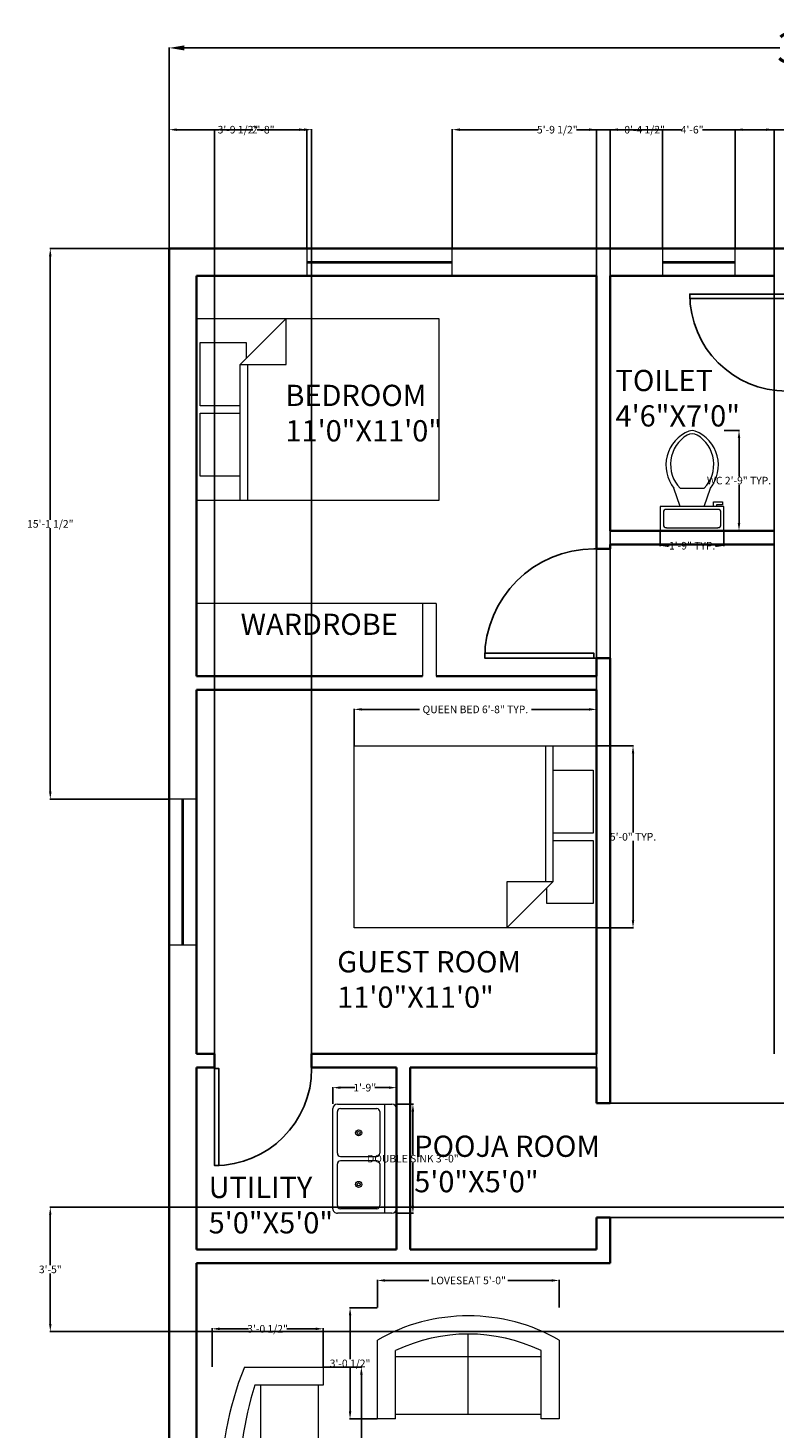
# Model space of a CAD drawing. Units: inches. Extents: x 481 to 2783, y 1975 to 3327.
# Tile 7 of 13: x 1328 to 1574, y 2866 to 3327. Entities that reach past the tile are written whole.
import ezdxf

# ---------------------------------------------------------------- set-up
doc = ezdxf.new("R2010")
doc.units = ezdxf.units.IN
doc.header["$MEASUREMENT"] = 0
for name, color, linetype, lineweight in [('A-ANNO-DIMS', 50, 'Continuous', 18), ('A-AREA-IDEN', 50, 'Continuous', 18), ('A-FLOR-CASE', 61, 'Continuous', 18), ('A-FLOR-FIXT', 61, 'Continuous', 18), ('A-FURN', 61, 'Continuous', 18), ('A-WALL', 40, 'Continuous', 35), ('DOORS', 10, 'Continuous', 25), ('WINDOWS', 220, 'Continuous', 20)]:
    doc.layers.add(name, color=color, linetype=linetype, lineweight=lineweight)
doc.styles.get("Standard").update_dxf_attribs({"font": 'arial.ttf'})
doc.dimstyles.get("Standard").update_dxf_attribs({"dimtxt": 2.5, "dimasz": 2.5, "dimexe": 0.18, "dimexo": 0.0625, "dimgap": 0.09, "dimtad": 0, "dimtih": 1, "dimtoh": 1, "dimzin": 0, "dimdsep": 46, "dimlunit": 3, "dimtxsty": 'Standard', "dimcen": 0.09, "dimadec": 0, "dimazin": 0, "dimtfac": 1, "dimtofl": 0, "dimtmove": 0, "dimatfit": 3, "dimfxl": 1, "dimtolj": 1, "dimtzin": 0, "dimarcsym": 0})

# ---------------------------------------------------------------- blocks, each defined once
blk = doc.blocks.new('*U2')
for p, q in [((0, 0), (0, -6)), ((40, 0), (40, -6))]:
    blk.add_line(p, q)
blk.add_lwpolyline([(0, 0), (0, 40), (1.75, 40), (1.75, 0)], close=True)
blk.add_arc((0, 0), 40, 0, 90)
blk = doc.blocks.new('Sink-double - 36 in top')
for p, q in [((-18, -4), (18, -4)), ((-0.75, -18.5), (-0.75, -6.5)), ((0.75, -6.5), (0.75, -18.5))]:
    blk.add_line(p, q)
for points in [[(-16.5, 0), (16.5, 0)], [(-18, -19.5), (-18, -1.5)], [(18, -1.5), (18, -19.5)], [(-16.5, -18.5), (-16.5, -6.5)], [(-15.5, -5.5), (-1.75, -5.5)], [(1.75, -5.5), (15.5, -5.5)], [(16.5, -6.5), (16.5, -18.5)], [(16.5, -21), (-16.5, -21)], [(-1.75, -19.5), (-15.5, -19.5)], [(15.5, -19.5), (1.75, -19.5)]]:
    blk.add_lwpolyline(points)
for centre, radius in [((-8.5, -12.5), 1), ((-8.5, -12.5), 0.5), ((8.5, -12.5), 1), ((8.5, -12.5), 0.5)]:
    blk.add_circle(centre, radius)
for centre, radius, start, end in [((-16.5, -1.5), 1.5, 90, 180), ((16.5, -1.5), 1.5, 0, 90), ((-15.5, -6.5), 1, 90, 180), ((-1.75, -6.5), 1, 0, 90), ((1.75, -6.5), 1, 90, 180), ((15.5, -6.5), 1, 0, 90), ((-16.5, -19.5), 1.5, 180, 270), ((-15.5, -18.5), 1, 180, 270), ((-1.75, -18.5), 1, 270, 0), ((1.75, -18.5), 1, 180, 270), ((15.5, -18.5), 1, 270, 0), ((16.5, -19.5), 1.5, 270, 0)]:
    blk.add_arc(centre, radius, start, end)
blk = doc.blocks.new('Sofa - Roundback 7 ft.')
for p, q in [((-12.00002, -32.4421), (-12.00003, -6.5971)), ((11.99997, -32.4421), (11.99998, -6.5971)), ((-36.000027, -34), (-36.000027, -11.4696)), ((-35.999844, -13.3819), (35.9998, -13.3819)), ((35.99998, -34), (35.99998, -11.4696)), ((-36.000027, -32.4421), (35.99998, -32.4421))]:
    blk.add_line(p, q)
for points in [[(-36.000027, -34), (-42.000027, -34), (-42.000027, -8)], [(41.99998, -8), (41.99998, -34), (35.99998, -34)]]:
    blk.add_lwpolyline(points)
for centre, radius, start, end in [((0, -114.25), 114.25, 68.43141, 111.5686), ((-0.00001, -127.1968), 121.1968, 72.72033, 107.2797)]:
    blk.add_arc(centre, radius, start, end)
blk = doc.blocks.new('Sofa - Roundback Loveseat 5 ft.')
for p, q in [((0, -32.44198), (0, -5.99998)), ((-24, -33.99998), (-24, -11.46958)), ((-23.9998, -13.38178), (23.99986, -13.38178)), ((24.00004, -33.99998), (24.00004, -11.46958)), ((-24, -32.44198), (24.00004, -32.44198))]:
    blk.add_line(p, q)
for points in [[(-24, -33.99998), (-30, -33.99998), (-30, -7.99998)], [(30.00004, -7.99998), (30.00004, -33.99998), (24.00004, -33.99998)]]:
    blk.add_lwpolyline(points)
for centre, radius, start, end in [((0, -60.24998), 60.24998, 60.13715, 119.8628), ((0, -61.38438), 55.38444, 64.32083, 115.6792)]:
    blk.add_arc(centre, radius, start, end)
blk = doc.blocks.new('Bed - Queen')
for p, q in [((0, -80.00003), (0, 0)), ((0, 0), (59.99999, 0)), ((59.99999, 0), (59.99999, -80.00003)), ((7.99999, -1.2), (28.79998, -1.2)), ((7.99999, -14.4), (7.99999, -1.2)), ((28.79998, -1.2), (28.79998, -14.4)), ((31.19999, -1.2), (51.99999, -1.2)), ((31.19999, -14.4), (31.19999, -1.2)), ((51.99999, -1.2), (51.99999, -16.4)), ((0, -14.4), (44.8, -14.4)), ((44.8, -16.8), (0, -16.8)), ((59.99999, -29.6), (44.8, -14.4)), ((44.8, -14.4), (44.8, -29.6)), ((51.99999, -16.4), (46.79936, -16.4)), ((44.8, -29.6), (59.99999, -29.6)), ((59.99999, -80.00003), (0, -80.00003))]:
    blk.add_line(p, q)
blk = doc.blocks.new('Toilet - top')
for p, q in [((9.5, -6), (9.5, -2)), ((-10, -8.5), (-8, -8.5)), ((-10, -9.5), (-10, -8.5)), ((-8, -8.5), (-8, -8)), ((-7, -8), (-7, -9.5)), ((-4, -8), (-6, -14)), ((4, -8), (6, -14)), ((-7, -9.5), (-10, -9.5)), ((4, -14), (-4, -14))]:
    blk.add_line(p, q)
blk.add_lwpolyline([(10.5, -8), (10.5, 0), (-10.5, 0), (-10.5, -8)], close=True)
for points in [[(-9.5, -2), (-9.5, -6)], [(8.5, -1), (-8.5, -1)], [(-8.5, -7), (8.5, -7)]]:
    blk.add_lwpolyline(points)
for centre, radius, start, end in [((-8.62, -1.88), 0.884, 81.8699, 188.1301), ((8.62, -1.88), 0.884, 351.8699, 98.1301), ((-8.62, -6.12), 0.884, 171.8699, 278.1301), ((8.62, -6.12), 0.884, 261.8699, 8.1301), ((3.52, -21.58), 12.17, 141.4691, 247.9714), ((4.2, -21.82), 11.33, 136.3677, 238.9468), ((-3.52, -21.58), 12.17, 292.0284, 38.5307), ((-4.2, -21.82), 11.33, 301.053, 43.6321), ((0, -27.88), 4, 245.7318, 294.2682), ((0, -29), 4, 254.8605, 285.1395)]:
    blk.add_arc(centre, radius, start, end)
blk = doc.blocks.new('*D24')
at = {"layer": 'A-ANNO-DIMS', "color": 0, "lineweight": -2, "transparency": 16777216}
for p, q in [((1374.44, 3254.39), (1374.44, 3320.66)), ((1379.44, 3320.48), (1575.87, 3320.48)), ((1789.44, 3320.48), (1593.01, 3320.48)), ((1794.44, 3254.39), (1794.44, 3320.66))]:
    blk.add_line(p, q, dxfattribs=at)
at = {"layer": 'A-ANNO-DIMS', "color": 0, "transparency": 16777216}
for points in [[(1379.44, 3321.31), (1379.44, 3319.65), (1374.44, 3320.48)], [(1789.44, 3321.31), (1789.44, 3319.65), (1794.44, 3320.48)]]:
    blk.add_solid(points, dxfattribs=at)
at = {"layer": 'Defpoints', "color": 0, "transparency": 16777216}
for p in [(1794.44, 3320.48), (1374.44, 3254.32), (1794.44, 3254.32)]:
    blk.add_point(p, dxfattribs=at)
at = {"layer": 'A-ANNO-DIMS', "color": 0, "transparency": 16777216, "insert": (1584.44, 3320.48), "char_height": 10, "attachment_point": 5}
blk.add_mtext("\\A1;35'", dxfattribs=at)
blk = doc.blocks.new('WIN-PLAN-48IN')
for p, q in [((0, 4.75), (48, 4.75)), ((0, 4.25), (48, 4.25))]:
    blk.add_line(p, q)
blk.add_lwpolyline([(0, 0), (48, 0), (48, 9), (0, 9)], close=True)
blk = doc.blocks.new('WIN-PLAN-24IN')
for p, q in [((0, 4.75), (24, 4.75)), ((0, 4.25), (24, 4.25))]:
    blk.add_line(p, q)
blk.add_lwpolyline([(0, 0), (24, 0), (24, 9), (0, 9)], close=True)
blk = doc.blocks.new('*D34')
at = {"layer": 'A-ANNO-DIMS', "color": 0, "lineweight": -2, "transparency": 16777216}
for p, q in [((1435.44, 3090.49), (1435.44, 3102.6)), ((1437.94, 3102.42), (1456.96, 3102.42)), ((1512.94, 3102.42), (1493.92, 3102.42)), ((1515.44, 3090.49), (1515.44, 3102.6))]:
    blk.add_line(p, q, dxfattribs=at)
at = {"layer": 'A-ANNO-DIMS', "color": 0, "transparency": 16777216}
for points in [[(1437.94, 3102.84), (1437.94, 3102.01), (1435.44, 3102.42)], [(1512.94, 3102.84), (1512.94, 3102.01), (1515.44, 3102.42)]]:
    blk.add_solid(points, dxfattribs=at)
at = {"layer": 'Defpoints', "color": 0, "transparency": 16777216}
for p in [(1515.44, 3102.42), (1435.44, 3090.42), (1515.44, 3090.42)]:
    blk.add_point(p, dxfattribs=at)
at = {"layer": 'A-ANNO-DIMS', "color": 0, "transparency": 16777216, "insert": (1475.44, 3102.42), "char_height": 2.5, "attachment_point": 5}
blk.add_mtext('\\A1;QUEEN BED 6\'-8" TYP.', dxfattribs=at)
blk = doc.blocks.new('*D35')
at = {"layer": 'A-ANNO-DIMS', "color": 0, "lineweight": -2, "transparency": 16777216}
for p, q in [((1515.5, 3090.42), (1527.62, 3090.42)), ((1527.44, 3087.92), (1527.44, 3061.79)), ((1527.44, 3032.92), (1527.44, 3059.06)), ((1515.5, 3030.42), (1527.62, 3030.42))]:
    blk.add_line(p, q, dxfattribs=at)
at = {"layer": 'A-ANNO-DIMS', "color": 0, "transparency": 16777216}
for points in [[(1527.02, 3087.92), (1527.85, 3087.92), (1527.44, 3090.42)], [(1527.02, 3032.92), (1527.85, 3032.92), (1527.44, 3030.42)]]:
    blk.add_solid(points, dxfattribs=at)
at = {"layer": 'Defpoints', "color": 0, "transparency": 16777216}
for p in [(1515.44, 3090.42), (1515.44, 3030.42), (1527.44, 3030.42)]:
    blk.add_point(p, dxfattribs=at)
at = {"layer": 'A-ANNO-DIMS', "color": 0, "transparency": 16777216, "insert": (1527.44, 3060.42), "char_height": 2.5, "attachment_point": 5}
blk.add_mtext('\\A1;5\'-0" TYP.', dxfattribs=at)
blk = doc.blocks.new('*D36')
at = {"layer": 'A-ANNO-DIMS', "color": 0, "lineweight": -2, "transparency": 16777216}
for p, q in [((1557.5, 3194.37), (1562.57, 3194.37)), ((1562.39, 3191.87), (1562.39, 3179.23)), ((1562.39, 3163.82), (1562.39, 3176.46)), ((1557.5, 3161.32), (1562.57, 3161.32))]:
    blk.add_line(p, q, dxfattribs=at)
at = {"layer": 'A-ANNO-DIMS', "color": 0, "transparency": 16777216}
for points in [[(1561.98, 3191.87), (1562.81, 3191.87), (1562.39, 3194.37)], [(1561.98, 3163.82), (1562.81, 3163.82), (1562.39, 3161.32)]]:
    blk.add_solid(points, dxfattribs=at)
at = {"layer": 'Defpoints', "color": 0, "transparency": 16777216}
for p in [(1557.44, 3194.37), (1557.44, 3161.32), (1562.39, 3161.32)]:
    blk.add_point(p, dxfattribs=at)
at = {"layer": 'A-ANNO-DIMS', "color": 0, "transparency": 16777216, "insert": (1562.39, 3177.85), "char_height": 2.5, "attachment_point": 5}
blk.add_mtext('\\A1;WC 2\'-9" TYP.', dxfattribs=at)
blk = doc.blocks.new('*D37')
at = {"layer": 'A-ANNO-DIMS', "color": 0, "lineweight": -2, "transparency": 16777216}
for p, q in [((1536.44, 3161.26), (1536.44, 3156.19)), ((1557.44, 3161.26), (1557.44, 3156.19)), ((1538.94, 3156.37), (1539.35, 3156.37)), ((1554.94, 3156.37), (1554.53, 3156.37))]:
    blk.add_line(p, q, dxfattribs=at)
at = {"layer": 'A-ANNO-DIMS', "color": 0, "transparency": 16777216}
for points in [[(1538.94, 3156.78), (1538.94, 3155.95), (1536.44, 3156.37)], [(1554.94, 3156.78), (1554.94, 3155.95), (1557.44, 3156.37)]]:
    blk.add_solid(points, dxfattribs=at)
at = {"layer": 'Defpoints', "color": 0, "transparency": 16777216}
for p in [(1536.44, 3161.32), (1557.44, 3161.32), (1536.44, 3156.37)]:
    blk.add_point(p, dxfattribs=at)
at = {"layer": 'A-ANNO-DIMS', "color": 0, "transparency": 16777216, "insert": (1546.94, 3156.37), "char_height": 2.5, "attachment_point": 5}
blk.add_mtext('\\A1;1\'-9" TYP.', dxfattribs=at)
blk = doc.blocks.new('*D40')
at = {"layer": 'A-ANNO-DIMS', "color": 0, "lineweight": -2, "transparency": 16777216}
for p, q in [((1449.5, 2972.32), (1455.02, 2972.32)), ((1454.84, 2969.82), (1454.84, 2955.71)), ((1454.84, 2938.82), (1454.84, 2952.94)), ((1449.5, 2936.32), (1455.02, 2936.32))]:
    blk.add_line(p, q, dxfattribs=at)
at = {"layer": 'A-ANNO-DIMS', "color": 0, "transparency": 16777216}
for points in [[(1454.42, 2969.82), (1455.25, 2969.82), (1454.84, 2972.32)], [(1454.42, 2938.82), (1455.25, 2938.82), (1454.84, 2936.32)]]:
    blk.add_solid(points, dxfattribs=at)
at = {"layer": 'Defpoints', "color": 0, "transparency": 16777216}
for p in [(1449.44, 2972.32), (1449.44, 2936.32), (1454.84, 2936.32)]:
    blk.add_point(p, dxfattribs=at)
at = {"layer": 'A-ANNO-DIMS', "color": 0, "transparency": 16777216, "insert": (1454.84, 2954.32), "char_height": 2.5, "attachment_point": 5}
blk.add_mtext('\\A1;DOUBLE SINK 3\'-0"', dxfattribs=at)
blk = doc.blocks.new('*D41')
at = {"layer": 'A-ANNO-DIMS', "color": 0, "lineweight": -2, "transparency": 16777216}
for p, q in [((1428.44, 2972.39), (1428.44, 2977.9)), ((1430.94, 2977.72), (1435.64, 2977.72)), ((1446.94, 2977.72), (1442.23, 2977.72)), ((1449.44, 2972.39), (1449.44, 2977.9))]:
    blk.add_line(p, q, dxfattribs=at)
at = {"layer": 'A-ANNO-DIMS', "color": 0, "transparency": 16777216}
for points in [[(1430.94, 2978.14), (1430.94, 2977.31), (1428.44, 2977.72)], [(1446.94, 2978.14), (1446.94, 2977.31), (1449.44, 2977.72)]]:
    blk.add_solid(points, dxfattribs=at)
at = {"layer": 'Defpoints', "color": 0, "transparency": 16777216}
for p in [(1449.44, 2977.72), (1428.44, 2972.32), (1449.44, 2972.32)]:
    blk.add_point(p, dxfattribs=at)
at = {"layer": 'A-ANNO-DIMS', "color": 0, "transparency": 16777216, "insert": (1438.94, 2977.72), "char_height": 2.5, "attachment_point": 5}
blk.add_mtext('\\A1;1\'-9"', dxfattribs=at)
blk = doc.blocks.new('*D44')
at = {"layer": 'A-ANNO-DIMS', "color": 0, "lineweight": -2, "transparency": 16777216}
for p, q in [((1425.31, 2885.62), (1438.02, 2885.62)), ((1437.84, 2883.12), (1437.84, 2845)), ((1437.84, 2804.12), (1437.84, 2842.24)), ((1425.31, 2801.62), (1438.02, 2801.62))]:
    blk.add_line(p, q, dxfattribs=at)
at = {"layer": 'A-ANNO-DIMS', "color": 0, "transparency": 16777216}
for points in [[(1437.43, 2883.12), (1438.26, 2883.12), (1437.84, 2885.62)], [(1437.43, 2804.12), (1438.26, 2804.12), (1437.84, 2801.62)]]:
    blk.add_solid(points, dxfattribs=at)
at = {"layer": 'Defpoints', "color": 0, "transparency": 16777216}
for p in [(1425.24, 2885.62), (1437.84, 2885.62), (1425.24, 2801.62)]:
    blk.add_point(p, dxfattribs=at)
at = {"layer": 'A-ANNO-DIMS', "color": 0, "transparency": 16777216, "insert": (1437.84, 2843.62), "char_height": 2.5, "attachment_point": 5}
blk.add_mtext('\\A1;SOFA 7\'-0"', dxfattribs=at)
blk = doc.blocks.new('*D45')
at = {"layer": 'A-ANNO-DIMS', "color": 0, "lineweight": -2, "transparency": 16777216}
for p, q in [((1388.58, 2885.68), (1388.58, 2898.4)), ((1425.24, 2885.68), (1425.24, 2898.4)), ((1391.08, 2898.22), (1400.59, 2898.22)), ((1422.74, 2898.22), (1413.23, 2898.22))]:
    blk.add_line(p, q, dxfattribs=at)
at = {"layer": 'A-ANNO-DIMS', "color": 0, "transparency": 16777216}
for points in [[(1391.08, 2898.64), (1391.08, 2897.8), (1388.58, 2898.22)], [(1422.74, 2898.64), (1422.74, 2897.8), (1425.24, 2898.22)]]:
    blk.add_solid(points, dxfattribs=at)
at = {"layer": 'Defpoints', "color": 0, "transparency": 16777216}
for p in [(1388.58, 2898.22), (1388.58, 2885.62), (1425.24, 2885.62)]:
    blk.add_point(p, dxfattribs=at)
at = {"layer": 'A-ANNO-DIMS', "color": 0, "transparency": 16777216, "insert": (1406.91, 2898.22), "char_height": 2.5, "attachment_point": 5}
blk.add_mtext('\\A1;3\'-0 1/2"', dxfattribs=at)
blk = doc.blocks.new('*D46')
at = {"layer": 'A-ANNO-DIMS', "color": 0, "lineweight": -2, "transparency": 16777216}
for p, q in [((1443.11, 2905.23), (1443.11, 2914.34)), ((1445.61, 2914.16), (1460.05, 2914.16)), ((1500.61, 2914.16), (1486.18, 2914.16)), ((1503.11, 2905.23), (1503.11, 2914.34))]:
    blk.add_line(p, q, dxfattribs=at)
at = {"layer": 'A-ANNO-DIMS', "color": 0, "transparency": 16777216}
for points in [[(1445.61, 2914.58), (1445.61, 2913.75), (1443.11, 2914.16)], [(1500.61, 2914.58), (1500.61, 2913.75), (1503.11, 2914.16)]]:
    blk.add_solid(points, dxfattribs=at)
at = {"layer": 'Defpoints', "color": 0, "transparency": 16777216}
for p in [(1503.11, 2914.16), (1443.11, 2905.16), (1503.11, 2905.16)]:
    blk.add_point(p, dxfattribs=at)
at = {"layer": 'A-ANNO-DIMS', "color": 0, "transparency": 16777216, "insert": (1473.11, 2914.16), "char_height": 2.5, "attachment_point": 5}
blk.add_mtext('\\A1;LOVESEAT 5\'-0"', dxfattribs=at)
blk = doc.blocks.new('*D47')
at = {"layer": 'A-ANNO-DIMS', "color": 0, "lineweight": -2, "transparency": 16777216}
for p, q in [((1443.05, 2905.16), (1433.93, 2905.16)), ((1434.11, 2902.66), (1434.11, 2888.21)), ((1434.11, 2871), (1434.11, 2885.45)), ((1443.05, 2868.5), (1433.93, 2868.5))]:
    blk.add_line(p, q, dxfattribs=at)
at = {"layer": 'A-ANNO-DIMS', "color": 0, "transparency": 16777216}
for points in [[(1433.7, 2902.66), (1434.53, 2902.66), (1434.11, 2905.16)], [(1433.7, 2871), (1434.53, 2871), (1434.11, 2868.5)]]:
    blk.add_solid(points, dxfattribs=at)
at = {"layer": 'Defpoints', "color": 0, "transparency": 16777216}
for p in [(1434.11, 2905.16), (1443.11, 2905.16), (1443.11, 2868.5)]:
    blk.add_point(p, dxfattribs=at)
at = {"layer": 'A-ANNO-DIMS', "color": 0, "transparency": 16777216, "insert": (1434.11, 2886.83), "char_height": 2.5, "attachment_point": 5}
blk.add_mtext('\\A1;3\'-0 1/2"', dxfattribs=at)
blk = doc.blocks.new('*D83')
at = {"layer": 'A-ANNO-DIMS', "color": 0, "lineweight": -2, "transparency": 16777216}
for p, q in [((1374.44, 3254.39), (1374.44, 3293.7)), ((1376.94, 3293.52), (1390.8, 3293.52)), ((1417.32, 3293.52), (1403.45, 3293.52)), ((1419.82, 3254.39), (1419.82, 3293.7))]:
    blk.add_line(p, q, dxfattribs=at)
at = {"layer": 'A-ANNO-DIMS', "color": 0, "transparency": 16777216}
for points in [[(1376.94, 3293.94), (1376.94, 3293.11), (1374.44, 3293.52)], [(1417.32, 3293.94), (1417.32, 3293.11), (1419.82, 3293.52)]]:
    blk.add_solid(points, dxfattribs=at)
at = {"layer": 'Defpoints', "color": 0, "transparency": 16777216}
for p in [(1419.82, 3293.52), (1374.44, 3254.32), (1419.82, 3254.32)]:
    blk.add_point(p, dxfattribs=at)
at = {"layer": 'A-ANNO-DIMS', "color": 0, "transparency": 16777216, "insert": (1397.13, 3293.52), "char_height": 2.5, "attachment_point": 5}
blk.add_mtext('\\A1;3\'-9 1/2"', dxfattribs=at)
blk = doc.blocks.new('*D84')
at = {"layer": 'A-ANNO-DIMS', "color": 0, "lineweight": -2, "transparency": 16777216}
for p, q in [((1467.82, 3254.39), (1467.82, 3293.7)), ((1470.32, 3293.52), (1496.15, 3293.52)), ((1534.63, 3293.52), (1508.8, 3293.52)), ((1537.13, 3254.39), (1537.13, 3293.7))]:
    blk.add_line(p, q, dxfattribs=at)
at = {"layer": 'A-ANNO-DIMS', "color": 0, "transparency": 16777216}
for points in [[(1470.32, 3293.94), (1470.32, 3293.11), (1467.82, 3293.52)], [(1534.63, 3293.94), (1534.63, 3293.11), (1537.13, 3293.52)]]:
    blk.add_solid(points, dxfattribs=at)
at = {"layer": 'Defpoints', "color": 0, "transparency": 16777216}
for p in [(1537.13, 3293.52), (1467.82, 3254.32), (1537.13, 3254.32)]:
    blk.add_point(p, dxfattribs=at)
at = {"layer": 'A-ANNO-DIMS', "color": 0, "transparency": 16777216, "insert": (1502.47, 3293.52), "char_height": 2.5, "attachment_point": 5}
blk.add_mtext('\\A1;5\'-9 1/2"', dxfattribs=at)
blk = doc.blocks.new('*D85')
at = {"layer": 'A-ANNO-DIMS', "color": 0, "lineweight": -2, "transparency": 16777216}
for p, q in [((1561.13, 3254.39), (1561.13, 3293.7)), ((1563.63, 3293.52), (1607.13, 3293.52)), ((1665.23, 3293.52), (1621.72, 3293.52)), ((1667.73, 3254.39), (1667.73, 3293.7))]:
    blk.add_line(p, q, dxfattribs=at)
at = {"layer": 'A-ANNO-DIMS', "color": 0, "transparency": 16777216}
for points in [[(1563.63, 3293.94), (1563.63, 3293.11), (1561.13, 3293.52)], [(1665.23, 3293.94), (1665.23, 3293.11), (1667.73, 3293.52)]]:
    blk.add_solid(points, dxfattribs=at)
at = {"layer": 'Defpoints', "color": 0, "transparency": 16777216}
for p in [(1667.73, 3293.52), (1561.13, 3254.32), (1667.73, 3254.32)]:
    blk.add_point(p, dxfattribs=at)
at = {"layer": 'A-ANNO-DIMS', "color": 0, "transparency": 16777216, "insert": (1614.43, 3293.52), "char_height": 2.5, "attachment_point": 5}
blk.add_mtext('\\A1;8\'-10 1/2"', dxfattribs=at)
blk = doc.blocks.new('*D92')
at = {"layer": 'A-ANNO-DIMS', "color": 0, "lineweight": -2, "transparency": 16777216}
for p, q in [((1374.38, 3254.32), (1335.06, 3254.32)), ((1335.24, 3251.82), (1335.24, 3164.96)), ((1335.24, 3075.32), (1335.24, 3162.19)), ((1374.38, 3072.82), (1335.06, 3072.82))]:
    blk.add_line(p, q, dxfattribs=at)
at = {"layer": 'A-ANNO-DIMS', "color": 0, "transparency": 16777216}
for points in [[(1334.82, 3251.82), (1335.65, 3251.82), (1335.24, 3254.32)], [(1334.82, 3075.32), (1335.65, 3075.32), (1335.24, 3072.82)]]:
    blk.add_solid(points, dxfattribs=at)
at = {"layer": 'Defpoints', "color": 0, "transparency": 16777216}
for p in [(1335.24, 3254.32), (1374.44, 3254.32), (1374.44, 3072.82)]:
    blk.add_point(p, dxfattribs=at)
at = {"layer": 'A-ANNO-DIMS', "color": 0, "transparency": 16777216, "insert": (1335.24, 3163.57), "char_height": 2.5, "attachment_point": 5}
blk.add_mtext('\\A1;15\'-1 1/2"', dxfattribs=at)
blk = doc.blocks.new('*D96')
at = {"layer": 'A-ANNO-DIMS', "color": 0, "lineweight": -2, "transparency": 16777216}
for p, q in [((1389.44, 2988.89), (1389.44, 3293.7)), ((1391.94, 3293.52), (1402, 3293.52)), ((1418.94, 3293.52), (1408.87, 3293.52)), ((1421.44, 2988.89), (1421.44, 3293.7))]:
    blk.add_line(p, q, dxfattribs=at)
at = {"layer": 'A-ANNO-DIMS', "color": 0, "transparency": 16777216}
for points in [[(1391.94, 3293.94), (1391.94, 3293.11), (1389.44, 3293.52)], [(1418.94, 3293.94), (1418.94, 3293.11), (1421.44, 3293.52)]]:
    blk.add_solid(points, dxfattribs=at)
at = {"layer": 'Defpoints', "color": 0, "transparency": 16777216}
for p in [(1421.44, 3293.52), (1389.44, 2988.82), (1421.44, 2988.82)]:
    blk.add_point(p, dxfattribs=at)
at = {"layer": 'A-ANNO-DIMS', "color": 0, "transparency": 16777216, "insert": (1405.44, 3293.52), "char_height": 2.5, "attachment_point": 5}
blk.add_mtext('\\A1;2\'-8"', dxfattribs=at)
blk = doc.blocks.new('*D97')
at = {"layer": 'A-ANNO-DIMS', "color": 0, "lineweight": -2, "transparency": 16777216}
for p, q in [((1520, 2972.64), (1833.82, 2972.64)), ((1833.64, 2970.14), (1833.64, 2955.16)), ((1833.64, 2937.42), (1833.64, 2952.39)), ((1520, 2934.92), (1833.82, 2934.92))]:
    blk.add_line(p, q, dxfattribs=at)
at = {"layer": 'A-ANNO-DIMS', "color": 0, "transparency": 16777216}
for points in [[(1833.22, 2970.14), (1834.05, 2970.14), (1833.64, 2972.64)], [(1833.22, 2937.42), (1834.05, 2937.42), (1833.64, 2934.92)]]:
    blk.add_solid(points, dxfattribs=at)
at = {"layer": 'Defpoints', "color": 0, "transparency": 16777216}
for p in [(1519.94, 2972.64), (1833.64, 2972.64), (1519.94, 2934.92)]:
    blk.add_point(p, dxfattribs=at)
at = {"layer": 'A-ANNO-DIMS', "color": 0, "transparency": 16777216, "insert": (1833.64, 2953.78), "char_height": 2.5, "attachment_point": 5}
blk.add_mtext('\\A1;3\'-1 1/2"', dxfattribs=at)
blk = doc.blocks.new('*D98')
at = {"layer": 'A-ANNO-DIMS', "color": 0, "lineweight": -2, "transparency": 16777216}
for p, q in [((1512.94, 3293.52), (1510.44, 3293.52)), ((1515.44, 2972.7), (1515.44, 3293.7)), ((1519.94, 2972.7), (1519.94, 3293.7)), ((1522.44, 3293.52), (1524.94, 3293.52))]:
    blk.add_line(p, q, dxfattribs=at)
at = {"layer": 'A-ANNO-DIMS', "color": 0, "transparency": 16777216}
for points in [[(1512.94, 3293.94), (1512.94, 3293.11), (1515.44, 3293.52)], [(1522.44, 3293.94), (1522.44, 3293.11), (1519.94, 3293.52)]]:
    blk.add_solid(points, dxfattribs=at)
at = {"layer": 'Defpoints', "color": 0, "transparency": 16777216}
for p in [(1519.94, 3293.52), (1515.44, 2972.64), (1519.94, 2972.64)]:
    blk.add_point(p, dxfattribs=at)
at = {"layer": 'A-ANNO-DIMS', "color": 0, "transparency": 16777216, "insert": (1531.26, 3293.52), "char_height": 2.5, "attachment_point": 5}
blk.add_mtext('\\A1;0\'-4 1/2"', dxfattribs=at)
blk = doc.blocks.new('*D103')
at = {"layer": 'A-ANNO-DIMS', "color": 0, "lineweight": -2, "transparency": 16777216}
for p, q in [((1761.38, 2938.3), (1335.06, 2938.3)), ((1335.24, 2935.8), (1335.24, 2919.18)), ((1335.24, 2899.82), (1335.24, 2916.45)), ((1761.38, 2897.32), (1335.06, 2897.32))]:
    blk.add_line(p, q, dxfattribs=at)
at = {"layer": 'A-ANNO-DIMS', "color": 0, "transparency": 16777216}
for points in [[(1334.82, 2935.8), (1335.65, 2935.8), (1335.24, 2938.3)], [(1334.82, 2899.82), (1335.65, 2899.82), (1335.24, 2897.32)]]:
    blk.add_solid(points, dxfattribs=at)
at = {"layer": 'Defpoints', "color": 0, "transparency": 16777216}
for p in [(1335.24, 2938.3), (1761.44, 2938.3), (1761.44, 2897.32)]:
    blk.add_point(p, dxfattribs=at)
at = {"layer": 'A-ANNO-DIMS', "color": 0, "transparency": 16777216, "insert": (1335.24, 2917.81), "char_height": 2.5, "attachment_point": 5}
blk.add_mtext('\\A1;3\'-5"', dxfattribs=at)
blk = doc.blocks.new('*D105')
at = {"layer": 'A-ANNO-DIMS', "color": 0, "lineweight": -2, "transparency": 16777216}
for p, q in [((1519.94, 2972.7), (1519.94, 3293.7)), ((1522.44, 3293.52), (1543.47, 3293.52)), ((1571.44, 3293.52), (1550.4, 3293.52)), ((1573.94, 2988.89), (1573.94, 3293.7))]:
    blk.add_line(p, q, dxfattribs=at)
at = {"layer": 'A-ANNO-DIMS', "color": 0, "transparency": 16777216}
for points in [[(1522.44, 3293.94), (1522.44, 3293.11), (1519.94, 3293.52)], [(1571.44, 3293.94), (1571.44, 3293.11), (1573.94, 3293.52)]]:
    blk.add_solid(points, dxfattribs=at)
at = {"layer": 'Defpoints', "color": 0, "transparency": 16777216}
for p in [(1573.94, 3293.52), (1573.94, 2988.82), (1519.94, 2972.64)]:
    blk.add_point(p, dxfattribs=at)
at = {"layer": 'A-ANNO-DIMS', "color": 0, "transparency": 16777216, "insert": (1546.94, 3293.52), "char_height": 2.5, "attachment_point": 5}
blk.add_mtext('\\A1;4\'-6"', dxfattribs=at)

msp = doc.modelspace()

# ---------------------------------------------------------------- linework, layer by layer
at = {"layer": 'A-FLOR-CASE'}
for p, q in [((1462.473, 3137.323), (1383.438, 3137.323)), ((1457.973, 3137.323), (1457.973, 3113.323)), ((1462.473, 3137.323), (1462.473, 3113.323))]:
    msp.add_line(p, q, dxfattribs=at)
at = {"layer": 'A-WALL'}
for p, q in [((1383.438, 3245.323), (1383.438, 3113.323)), ((1515.438, 3245.323), (1383.438, 3245.323)), ((1515.438, 3245.323), (1515.438, 3155.323)), ((1519.938, 3245.323), (1519.938, 3161.323)), ((1573.938, 3245.323), (1519.938, 3245.323)), ((1573.938, 3161.323), (1519.938, 3161.323)), ((1573.938, 3156.823), (1519.938, 3156.823)), ((1519.938, 3156.823), (1519.938, 3155.323)), ((1515.438, 3155.323), (1519.938, 3155.323)), ((1515.438, 3119.323), (1519.938, 3119.323)), ((1515.438, 3119.323), (1515.438, 3113.323)), ((1519.938, 3119.323), (1519.938, 2972.637)), ((1457.973, 3113.323), (1383.438, 3113.323)), ((1515.438, 3113.323), (1462.473, 3113.323)), ((1515.438, 3108.823), (1383.438, 3108.823)), ((1383.438, 3108.823), (1383.438, 2988.823)), ((1515.438, 3108.823), (1515.438, 2988.823)), ((1389.438, 2988.823), (1383.438, 2988.823)), ((1389.438, 2988.823), (1389.438, 2984.323)), ((1515.438, 2988.823), (1421.438, 2988.823)), ((1421.438, 2988.823), (1421.438, 2984.323)), ((1383.438, 2984.323), (1383.438, 2924.323)), ((1389.438, 2984.323), (1383.438, 2984.323)), ((1449.438, 2984.323), (1421.438, 2984.323)), ((1449.438, 2984.323), (1449.438, 2924.323)), ((1515.438, 2984.323), (1453.938, 2984.323)), ((1453.938, 2984.323), (1453.938, 2924.323)), ((1515.438, 2984.323), (1515.438, 2972.637)), ((1515.438, 2972.637), (1519.938, 2972.637)), ((1515.438, 2934.918), (1519.938, 2934.918)), ((1515.438, 2934.918), (1515.438, 2924.323)), ((1519.938, 2934.918), (1519.938, 2919.823)), ((1449.438, 2924.323), (1383.438, 2924.323)), ((1515.438, 2924.323), (1453.938, 2924.323)), ((1519.938, 2919.823), (1383.438, 2919.823)), ((1383.438, 2919.823), (1383.438, 2760.823))]:
    msp.add_line(p, q, dxfattribs=at)
msp.add_lwpolyline([(1794.438, 2864.323), (1794.438, 3254.323), (1374.438, 3254.323), (1374.438, 2654.323), (1582.938, 2654.323)], dxfattribs=at)

# ---------------------------------------------------------------- block references
at = {"layer": 'A-FLOR-FIXT'}
for name, p, rotation in [('Toilet - top', (1546.938, 3161.323), 180), ('Sink-double - 36 in top', (1449.438, 2954.323), 270)]:
    msp.add_blockref(name, p, dxfattribs=dict(at, rotation=rotation))
at = {"layer": 'A-FURN'}
for name, p, rotation in [('Bed - Queen', (1383.438, 3171.323), 89.99999999999999), ('Bed - Queen', (1515.438, 3090.423), 270), ('Sofa - Roundback 7 ft.', (1391.243, 2843.619), 90)]:
    msp.add_blockref(name, p, dxfattribs=dict(at, rotation=rotation))
msp.add_blockref('Sofa - Roundback Loveseat 5 ft.', (1473.114, 2902.497), dxfattribs=at)
at = {"layer": 'DOORS'}
for p, xscale, yscale, zscale, rotation in [((1578.138, 3239.323), -0.8, 0.8, 0.8, 90), ((1514.538, 3119.323), 0.9, 0.9, 0.9, 90), ((1389.438, 2984.023), -0.8, 0.8, 0.8, 180)]:
    msp.add_blockref('*U2', p, dxfattribs=dict(at, xscale=xscale, yscale=yscale, zscale=zscale, rotation=rotation))
at = {"layer": 'WINDOWS'}
for name, p in [('WIN-PLAN-48IN', (1419.821, 3245.323)), ('WIN-PLAN-24IN', (1537.126, 3245.323))]:
    msp.add_blockref(name, p, dxfattribs=at)
at = {"layer": 'WINDOWS', "rotation": 89.99999999999991}
msp.add_blockref('WIN-PLAN-48IN', (1383.438, 3024.823), dxfattribs=at)

# ---------------------------------------------------------------- texts
at = {"layer": 'A-AREA-IDEN', "char_height": 7, "attachment_point": 1}
for s, width, insert in [('TOILET\\P4\'6"X7\'0"', 43.33543, (1521.669, 3214.343)), ('BEDROOM\\P11\'0"X11\'0"', 43.33543, (1412.806, 3209.427)), ('WARDROBE', 43.33543, (1398, 3133.977)), ('GUEST ROOM\\P11\'0"X11\'0"', 67.28168, (1429.878, 3022.724)), ('POOJA ROOM\\P5\'0"X5\'0"', 69.01413, (1455.272, 2961.907)), ('UTILITY\\P5\'0"X5\'0"', 43.33543, (1387.473, 2948.338))]:
    msp.add_mtext_dynamic_manual_height_columns(s, width=width, gutter_width=1, heights=[0], dxfattribs=dict(at, insert=insert))

# ---------------------------------------------------------------- dimensions: what is measured, and where the dimension line sits
at = {"layer": 'A-ANNO-DIMS'}
dim = msp.add_aligned_dim(p1=(1374.438, 3254.323), p2=(1794.438, 3254.323), distance=66.156, dimstyle='Standard', override={"dimtxt": 10, "dimasz": 5, "dimclrd": 0, "dimclre": 0, "dimclrt": 0}, dxfattribs=at)
dim.commit()
dim.dimension.update_dxf_attribs({"geometry": '*D24', "text_midpoint": (1584.438, 3320.479)})
for base, p1, p2, picture, middle in [((1419.821, 3293.523), (1374.438, 3254.323), (1419.821, 3254.323), '*D83', (1397.129, 3293.523)), ((1537.126, 3293.523), (1467.821, 3254.323), (1537.126, 3254.323), '*D84', (1502.473, 3293.523)), ((1519.938, 3293.523), (1515.438, 2972.637), (1519.938, 2972.637), '*D98', (1531.263, 3293.523)), ((1667.726, 3293.523), (1561.126, 3254.323), (1667.726, 3254.323), '*D85', (1614.426, 3293.523)), ((1421.438, 3293.523), (1389.438, 2988.823), (1421.438, 2988.823), '*D96', (1405.438, 3293.523)), ((1573.938, 3293.523), (1519.938, 2972.637), (1573.938, 2988.823), '*D105', (1546.938, 3293.523)), ((1449.438, 2977.723), (1428.438, 2972.323), (1449.438, 2972.323), '*D41', (1438.938, 2977.723))]:
    dim = msp.add_linear_dim(base=base, p1=p1, p2=p2, dimstyle='Standard', override={"dimdec": 1, "dimlfac": 1, "dimrnd": 0, "dimzin": 1, "dimdsep": 46, "dimlunit": 4, "dimfrac": 2}, dxfattribs=at)
    dim.commit()
    dim.dimension.update_dxf_attribs({"geometry": picture, "text_midpoint": middle})
for base, p1, p2, angle, picture, middle in [((1335.238, 3254.323), (1374.438, 3072.823), (1374.438, 3254.323), 90, '*D92', (1335.238, 3163.573)), ((1833.638, 2972.637), (1519.938, 2934.918), (1519.938, 2972.637), 90, '*D97', (1833.638, 2953.778)), ((1335.238, 2938.303), (1761.438, 2897.323), (1761.438, 2938.303), 90, '*D103', (1335.238, 2917.813)), ((1434.114, 2905.164), (1443.114, 2868.497), (1443.114, 2905.164), 90, '*D47', (1434.114, 2886.831)), ((1388.577, 2898.219), (1425.243, 2885.619), (1388.577, 2885.619), 180, '*D45', (1406.91, 2898.219))]:
    dim = msp.add_linear_dim(base=base, p1=p1, p2=p2, angle=angle, dimstyle='Standard', override={"dimdec": 1, "dimlfac": 1, "dimrnd": 0, "dimzin": 1, "dimdsep": 46, "dimlunit": 4, "dimfrac": 2}, dxfattribs=at)
    dim.commit()
    dim.dimension.update_dxf_attribs({"geometry": picture, "text_midpoint": middle})
for base, p1, p2, angle, text, picture, middle in [((1562.395, 3161.323), (1557.438, 3194.369), (1557.438, 3161.323), 270, 'WC <> TYP.', '*D36', (1562.395, 3177.846)), ((1536.438, 3156.366), (1557.438, 3161.323), (1536.438, 3161.323), 180, '<> TYP.', '*D37', (1546.938, 3156.366)), ((1527.438, 3030.423), (1515.438, 3090.423), (1515.438, 3030.423), 270, '<> TYP.', '*D35', (1527.438, 3060.423)), ((1454.838, 2936.323), (1449.438, 2972.323), (1449.438, 2936.323), 270, 'DOUBLE SINK <>', '*D40', (1454.838, 2954.323)), ((1437.843, 2885.619), (1425.243, 2801.619), (1425.243, 2885.619), 90, 'SOFA <>', '*D44', (1437.843, 2843.619))]:
    dim = msp.add_linear_dim(base=base, p1=p1, p2=p2, angle=angle, text=text, dimstyle='Standard', override={"dimdec": 1, "dimlfac": 1, "dimrnd": 0, "dimzin": 1, "dimdsep": 46, "dimlunit": 4, "dimfrac": 2}, dxfattribs=at)
    dim.commit()
    dim.dimension.update_dxf_attribs({"geometry": picture, "text_midpoint": middle})
for base, p1, p2, text, picture, middle in [((1515.438, 3102.423), (1435.438, 3090.423), (1515.438, 3090.423), 'QUEEN BED <> TYP.', '*D34', (1475.438, 3102.423)), ((1503.114, 2914.164), (1443.114, 2905.164), (1503.114, 2905.164), 'LOVESEAT <>', '*D46', (1473.114, 2914.164))]:
    dim = msp.add_linear_dim(base=base, p1=p1, p2=p2, text=text, dimstyle='Standard', override={"dimdec": 1, "dimlfac": 1, "dimrnd": 0, "dimzin": 1, "dimdsep": 46, "dimlunit": 4, "dimfrac": 2}, dxfattribs=at)
    dim.commit()
    dim.dimension.update_dxf_attribs({"geometry": picture, "text_midpoint": middle})

doc.saveas('drawing.dxf')
